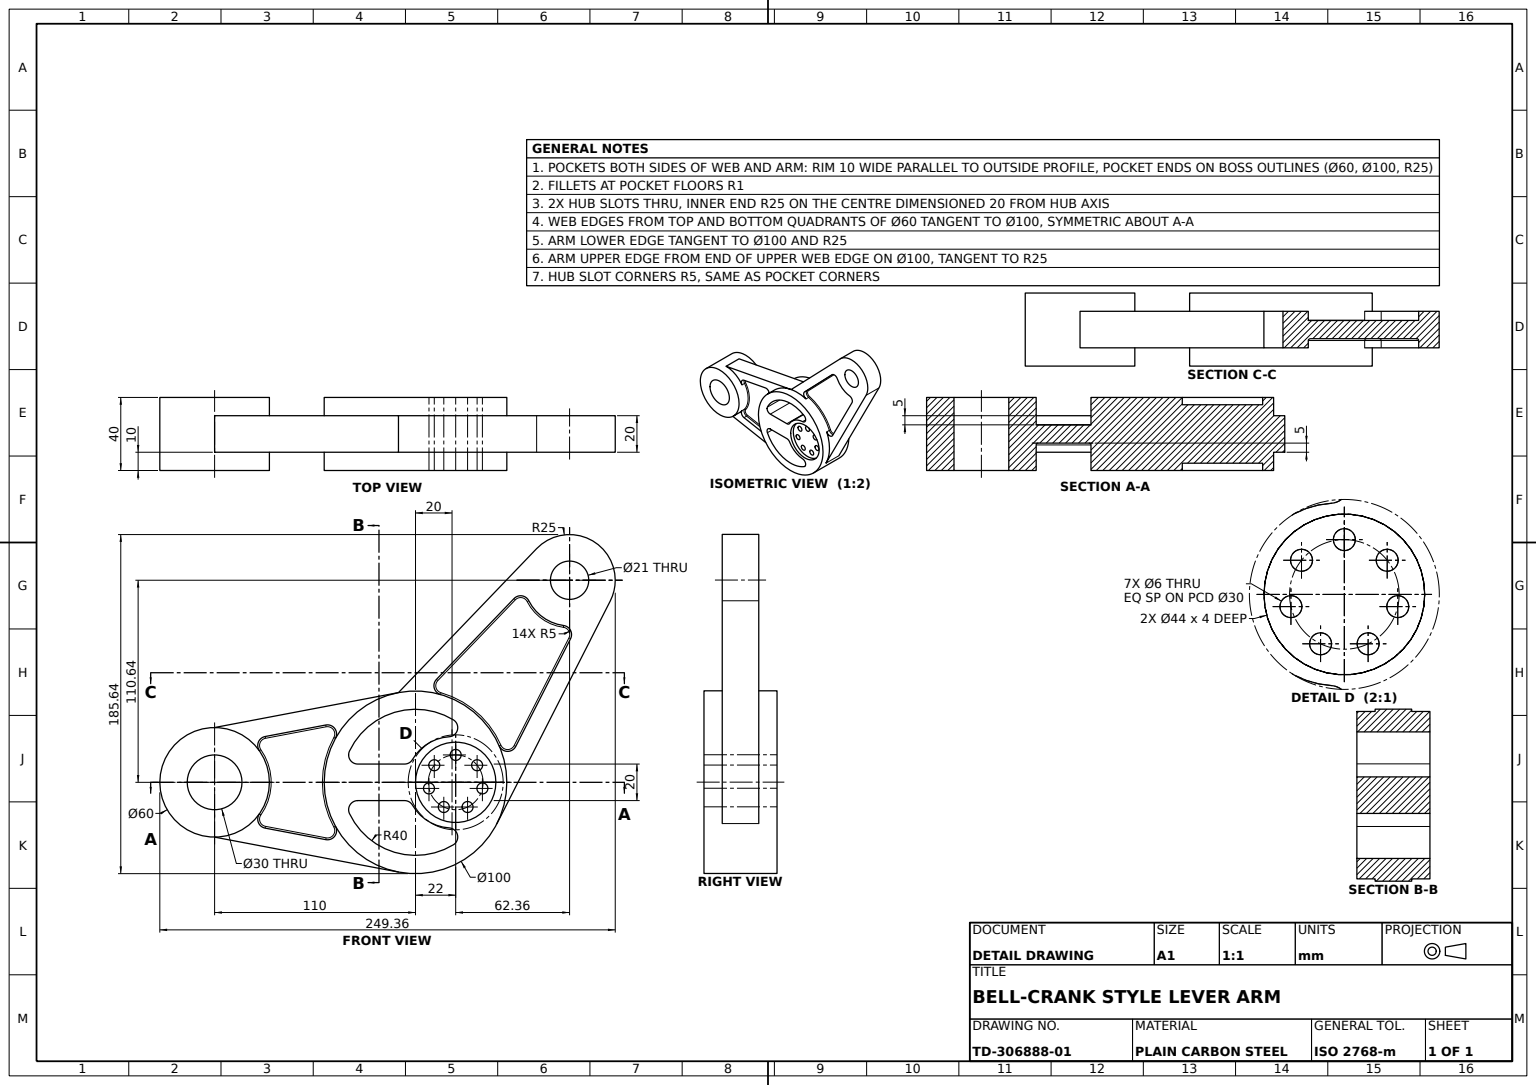
from build123d import *

# Parameters (mm, degrees)
LEVER_BODY_PROFILE_R      = 50
LEVER_BODY_DEPTH          = 40
FRONT_POCKET_PROFILE_R    = 22
FRONT_POCKET_PROFILE_R_2  = 3
FRONT_POCKET_4MM_DEPTH    = 4
HUB_THROUGH_CUT_PROFILE_R = 3
HUB_THROUGH_CUT_DEPTH     = 44
REAR_START                = -4
REAR_POCKET_PROFILE_R     = 22
REAR_POCKET_PROFILE_R_2   = 3
REAR_POCKET_4MM_DEPTH     = 4
ARM_BOSS_PROFILE_R        = 30
ARM_BOSS_PROFILE_R_2      = 15
ARM_BOSS_DEPTH            = 40
WEB_ARM_PROFILE_R         = 25
WEB_ARM_PROFILE_R_2       = 10.5
TRIANGULAR_WEB_ARM_DEPTH  = 40
FRONT_HUB_BOSS_DEPTH      = 10
REAR_HUB_FLANGE_DEPTH     = 5
HUB_EDGE_FILLET_R1_A_R    = 1
HUB_EDGE_FILLET_R1_B_R    = 1
WEB_ARM_CUT_A_PROFILE_R   = 25
WEB_ARM_CUT_A_PROFILE_R_2 = 10.5
WEB_ARM_CUT_A_DEPTH       = 10
WEB_START                 = -10
WEB_ARM_CUT_B_PROFILE_R   = 25
WEB_ARM_CUT_B_PROFILE_R_2 = 10.5
WEB_ARM_CUT_B_DEPTH       = 10


with BuildPart() as part:
    # Lever Body Profile → Lever Body (new body)
    with BuildSketch(Plane.XY):
        Circle(LEVER_BODY_PROFILE_R)
        with BuildLine():
            Line((-5.980762114, 10), (-31.622776602, 10))
            ThreePointArc((-31.622776602, 10), (-35.848547875, 12.327387581), (-36.140316116, 17.142857143))
            ThreePointArc((-36.140316116, 17.142857143), (-11.505936436, 38.309443049), (20.714285714, 34.218684477))
            ThreePointArc((20.714285714, 34.218684477), (22.980616225, 28.748457023), (18.4375, 24.951124098))
            ThreePointArc((18.4375, 24.951124098), (6.829197706, 21.249234503), (-1.650635095, 12.5))
            ThreePointArc((-1.650635095, 12.5), (-3.480762114, 10.669872981), (-5.980762114, 10))
        make_face(mode=Mode.SUBTRACT)
        with BuildLine():
            Line((-5.980762114, -10), (-31.622776602, -10))
            ThreePointArc((-31.622776602, -10), (-35.848547875, -12.327387581), (-36.140316116, -17.142857143))
            ThreePointArc((-36.140316116, -17.142857143), (-11.505936436, -38.309443049), (20.714285714, -34.218684477))
            ThreePointArc((20.714285714, -34.218684477), (22.980616225, -28.748457023), (18.4375, -24.951124098))
            ThreePointArc((18.4375, -24.951124098), (6.829197706, -21.249234503), (-1.650635095, -12.5))
            ThreePointArc((-1.650635095, -12.5), (-3.480762114, -10.669872981), (-5.980762114, -10))
        make_face(mode=Mode.SUBTRACT)
    extrude(amount=LEVER_BODY_DEPTH)

    # Front Pocket Profile → Front Pocket 4mm (cut)
    with BuildSketch(Plane.XY.offset(40)):
        with Locations((22, 0)):
            Circle(FRONT_POCKET_PROFILE_R)
        with Locations((22, 15)):
            Circle(FRONT_POCKET_PROFILE_R_2, mode=Mode.SUBTRACT)
        with Locations((33.727472237, 9.352347028)):
            Circle(FRONT_POCKET_PROFILE_R_2, mode=Mode.SUBTRACT)
        with Locations((36.623918683, -3.337814009)):
            Circle(FRONT_POCKET_PROFILE_R_2, mode=Mode.SUBTRACT)
        with Locations((28.508256087, -13.514533019)):
            Circle(FRONT_POCKET_PROFILE_R_2, mode=Mode.SUBTRACT)
        with Locations((15.491743913, -13.514533019)):
            Circle(FRONT_POCKET_PROFILE_R_2, mode=Mode.SUBTRACT)
        with Locations((7.376081317, -3.337814009)):
            Circle(FRONT_POCKET_PROFILE_R_2, mode=Mode.SUBTRACT)
        with Locations((10.272527763, 9.352347028)):
            Circle(FRONT_POCKET_PROFILE_R_2, mode=Mode.SUBTRACT)
    extrude(amount=-FRONT_POCKET_4MM_DEPTH, mode=Mode.SUBTRACT)

    # Hub Through Cut Profile → Hub Through Cut (cut)
    with BuildSketch(Plane.XY.offset(40)):
        with Locations((22, 15)):
            Circle(HUB_THROUGH_CUT_PROFILE_R)
        with Locations((33.727472237, 9.352347028)):
            Circle(HUB_THROUGH_CUT_PROFILE_R)
        with Locations((36.623918683, -3.337814009)):
            Circle(HUB_THROUGH_CUT_PROFILE_R)
        with Locations((28.508256087, -13.514533019)):
            Circle(HUB_THROUGH_CUT_PROFILE_R)
        with Locations((15.491743913, -13.514533019)):
            Circle(HUB_THROUGH_CUT_PROFILE_R)
        with Locations((7.376081317, -3.337814009)):
            Circle(HUB_THROUGH_CUT_PROFILE_R)
        with Locations((10.272527763, 9.352347028)):
            Circle(HUB_THROUGH_CUT_PROFILE_R)
    extrude(amount=-HUB_THROUGH_CUT_DEPTH, mode=Mode.SUBTRACT)

    # Rear Pocket Profile → Rear Pocket 4mm (cut)
    with BuildSketch(Plane(origin=(0, 0, 0), x_dir=(-1, 0, 0), z_dir=(0, 0, -1)).offset(REAR_START)):
        with Locations(Location((-22, 0, 0), (0, 0, 180))):
            Circle(REAR_POCKET_PROFILE_R)
        with Locations(Location((-22, 15, 0), (0, 0, 180))):
            Circle(REAR_POCKET_PROFILE_R_2, mode=Mode.SUBTRACT)
        with Locations(Location((-10.272527763, 9.352347028, 0), (0, 0, 180))):
            Circle(REAR_POCKET_PROFILE_R_2, mode=Mode.SUBTRACT)
        with Locations(Location((-7.376081317, -3.337814009, 0), (0, 0, 180))):
            Circle(REAR_POCKET_PROFILE_R_2, mode=Mode.SUBTRACT)
        with Locations(Location((-15.491743913, -13.514533019, 0), (0, 0, 180))):
            Circle(REAR_POCKET_PROFILE_R_2, mode=Mode.SUBTRACT)
        with Locations(Location((-28.508256087, -13.514533019, 0), (0, 0, 180))):
            Circle(REAR_POCKET_PROFILE_R_2, mode=Mode.SUBTRACT)
        with Locations(Location((-36.623918683, -3.337814009, 0), (0, 0, 180))):
            Circle(REAR_POCKET_PROFILE_R_2, mode=Mode.SUBTRACT)
        with Locations(Location((-33.727472237, 9.352347028, 0), (0, 0, 180))):
            Circle(REAR_POCKET_PROFILE_R_2, mode=Mode.SUBTRACT)
    extrude(amount=REAR_POCKET_4MM_DEPTH, mode=Mode.SUBTRACT)



with BuildPart() as body_2:
    # Arm Boss Profile → Arm Boss (new body)
    with BuildSketch(Plane.XY.offset(40)):
        with Locations((-110, 0)):
            Circle(ARM_BOSS_PROFILE_R)
        with Locations((-110, 0)):
            Circle(ARM_BOSS_PROFILE_R_2, mode=Mode.SUBTRACT)
    extrude(amount=-ARM_BOSS_DEPTH)


with BuildPart() as body_3:
    # Web Arm Profile → Triangular Web Arm (new body)
    with BuildSketch(Plane.XY.offset(40)):
        with Locations((84.359013574, 110.636130744)):
            Circle(WEB_ARM_PROFILE_R)
        with Locations((84.359013574, 110.636130744)):
            Circle(WEB_ARM_PROFILE_R_2, mode=Mode.SUBTRACT)
    extrude(amount=-TRIANGULAR_WEB_ARM_DEPTH)


with BuildPart() as part_1:
    add(part.part)

    add(body_2.part)  # Front Hub Boss merges body 2

    add(body_3.part)  # Front Hub Boss merges body 3
    # Front Hub Boss Profile → Front Hub Boss (add, symmetric)
    with BuildSketch(Plane.XY.offset(20)):
        with BuildLine():
            Line((-9.330441424, 49.121714779), (-110, 30))
            ThreePointArc((-110, 30), (-96.189540691, 26.632146246), (-85.479855197, 17.284747578))
            ThreePointArc((-85.479855197, 17.284747578), (-86.028032441, 22.041171589), (-82.326208539, 25.077710319))
            Line((-82.326208539, 25.077710319), (-49.145510288, 31.38022974))
            ThreePointArc((-49.145510288, 31.38022974), (-44.167091223, 29.4065854), (-43.829514678, 24.061871148))
            ThreePointArc((-43.829514678, 24.061871148), (-29.385271377, 40.453749222), (-9.330441424, 49.121714779))
        make_face()
        with BuildLine():
            ThreePointArc((-82.326208539, -25.077710319), (-86.028032441, -22.041171589), (-85.479855197, -17.284747578))
            ThreePointArc((-85.479855197, -17.284747578), (-96.189540691, -26.632146246), (-110, -30))
            Line((-110, -30), (-9.330441424, -49.121714779))
            ThreePointArc((-9.330441424, -49.121714779), (-29.385271377, -40.453749222), (-43.829514678, -24.061871148))
            ThreePointArc((-43.829514678, -24.061871148), (-44.167091223, -29.4065854), (-49.145510288, -31.38022974))
            Line((-49.145510288, -31.38022974), (-82.326208539, -25.077710319))
        make_face()
        with BuildLine():
            Line((66.322063718, 127.947064858), (-9.330441424, 49.121714779))
            ThreePointArc((-9.330441424, 49.121714779), (2.249613331, 49.949366761), (13.708384523, 48.084095019))
            ThreePointArc((13.708384523, 48.084095019), (10.252590563, 51.587276744), (11.471833004, 56.354691343))
            Line((11.471833004, 56.354691343), (53.95175742, 100.616211925))
            ThreePointArc((53.95175742, 100.616211925), (58.303283523, 102.098341173), (62.025791755, 99.401042709))
            ThreePointArc((62.025791755, 99.401042709), (59.637433216, 114.356811406), (66.322063718, 127.947064858))
        make_face()
        with BuildLine():
            ThreePointArc((54.892353403, 19.667982557), (50.284966201, 16.9381636), (45.851155545, 19.941703417))
            ThreePointArc((45.851155545, 19.941703417), (48.951801689, 10.184356208), (50, 0))
            ThreePointArc((50, 0), (48.621194719, -11.661021572), (44.560823036, -22.67891202))
            Line((44.560823036, -22.67891202), (106.639425092, 99.296674734))
            ThreePointArc((106.639425092, 99.296674734), (96.00405542, 88.513902095), (81.094875761, 85.850138645))
            ThreePointArc((81.094875761, 85.850138645), (84.866493928, 83.221948595), (84.898130502, 78.625049023))
            Line((84.898130502, 78.625049023), (54.892353403, 19.667982557))
        make_face()
    extrude(amount=FRONT_HUB_BOSS_DEPTH, both=True)

    # Rear Hub Flange Profile → Rear Hub Flange (add, symmetric)
    with BuildSketch(Plane.XY.offset(20)):
        with BuildLine():
            Line((-82.326208539, 25.077710319), (-49.145510288, 31.38022974))
            ThreePointArc((-49.145510288, 31.38022974), (-44.167091223, 29.4065854), (-43.829514678, 24.061871148))
            ThreePointArc((-43.829514678, 24.061871148), (-50, 0), (-43.829514678, -24.061871148))
            ThreePointArc((-43.829514678, -24.061871148), (-44.167091223, -29.4065854), (-49.145510288, -31.38022974))
            Line((-49.145510288, -31.38022974), (-82.326208539, -25.077710319))
            ThreePointArc((-82.326208539, -25.077710319), (-86.028032441, -22.041171589), (-85.479855197, -17.284747578))
            ThreePointArc((-85.479855197, -17.284747578), (-80, 0), (-85.479855197, 17.284747578))
            ThreePointArc((-85.479855197, 17.284747578), (-86.028032441, 22.041171589), (-82.326208539, 25.077710319))
        make_face()
        with BuildLine():
            Line((11.471833004, 56.354691343), (53.95175742, 100.616211925))
            ThreePointArc((53.95175742, 100.616211925), (58.303283523, 102.098341173), (62.025791755, 99.401042709))
            ThreePointArc((62.025791755, 99.401042709), (69.877544198, 90.257537939), (81.094875761, 85.850138645))
            ThreePointArc((81.094875761, 85.850138645), (84.866493928, 83.221948595), (84.898130502, 78.625049023))
            Line((84.898130502, 78.625049023), (54.892353403, 19.667982557))
            ThreePointArc((54.892353403, 19.667982557), (50.284966201, 16.9381636), (45.851155545, 19.941703417))
            ThreePointArc((45.851155545, 19.941703417), (32.936806988, 37.61870207), (13.708384523, 48.084095019))
            ThreePointArc((13.708384523, 48.084095019), (10.252590563, 51.587276744), (11.471833004, 56.354691343))
        make_face()
    extrude(amount=REAR_HUB_FLANGE_DEPTH, both=True)

    # Hub Edge Fillet R1 A
    hub_edge_fillet_r1_a_edges = [part_1.edges().sort_by_distance(p)[0] for p in [
        (-81.402759363, 9.066301779, 25),
        (-86.028032441, -22.041171589, 25),
        (-65.735859413, -28.22897003, 25),
        (-44.167091223, -29.4065854, 25),
        (-50, 0, 25),
        (-44.167091223, 29.4065854, 25),
        (-65.735859413, 28.22897003, 25),
        (-86.028032441, 22.041171589, 25),
    ]]
    fillet(hub_edge_fillet_r1_a_edges, radius=HUB_EDGE_FILLET_R1_A_R)

    # Hub Edge Fillet R1 B
    hub_edge_fillet_r1_b_edges = [part_1.edges().sort_by_distance(p)[0] for p in [
        (10.252590563, 51.587276744, 25),
        (32.936806988, 37.61870207, 25),
        (50.284966201, 16.9381636, 25),
        (69.895241952, 49.14651579, 25),
        (84.866493928, 83.221948595, 25),
        (69.877544198, 90.257537939, 25),
        (58.303283523, 102.098341173, 25),
        (32.711795212, 78.485451634, 25),
    ]]
    fillet(hub_edge_fillet_r1_b_edges, radius=HUB_EDGE_FILLET_R1_B_R)

    # Web Arm Cut A Profile → Web Arm Cut A (cut)
    with BuildSketch(Plane.XY.offset(40)):
        with Locations((84.359013574, 110.636130744)):
            Circle(WEB_ARM_CUT_A_PROFILE_R)
        with Locations((84.359013574, 110.636130744)):
            Circle(WEB_ARM_CUT_A_PROFILE_R_2, mode=Mode.SUBTRACT)
    extrude(amount=-WEB_ARM_CUT_A_DEPTH, mode=Mode.SUBTRACT)

    # Web Arm Cut B Profile → Web Arm Cut B (cut)
    with BuildSketch(Plane(origin=(0, 0, 0), x_dir=(-1, 0, 0), z_dir=(0, 0, -1)).offset(WEB_START)):
        with Locations((-84.359013574, 110.636130744)):
            Circle(WEB_ARM_CUT_B_PROFILE_R)
        with Locations(Location((-84.359013574, 110.636130744, 0), (0, 0, 180))):
            Circle(WEB_ARM_CUT_B_PROFILE_R_2, mode=Mode.SUBTRACT)
    extrude(amount=WEB_ARM_CUT_B_DEPTH, mode=Mode.SUBTRACT)


solid = part_1.part
